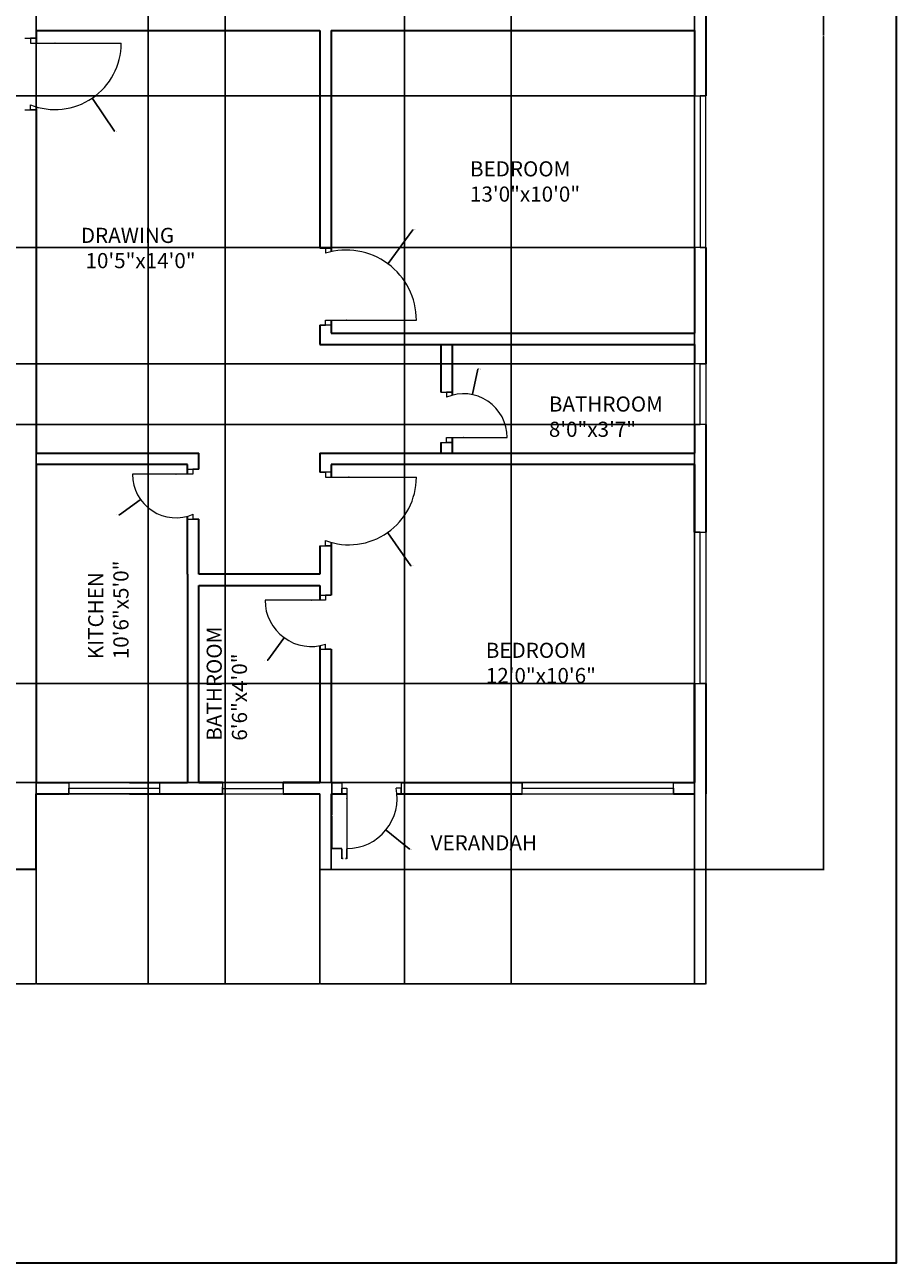
# Model space of a CAD drawing. Units: inches. Extents: x 1831 to 2867, y 1605 to 2524.
# Tile 6 of 7: x 2522 to 2867, y 1605 to 2096. Entities that reach past the tile are written whole.
import ezdxf

# ---------------------------------------------------------------- set-up
doc = ezdxf.new("R2010")
doc.units = ezdxf.units.IN
for name, color, linetype, lineweight in [('A-ANNO-DIMS', 2, 'Continuous', 18), ('A-ANNO-TTLB', 7, 'Continuous', 35), ('A-AREA-IDEN', 7, 'Continuous', 18), ('A-DOOR', 11, 'Continuous', 18), ('A-FLOR-BALC', 7, 'Continuous', 25), ('A-GLAZ', 121, 'Continuous', 18), ('A-WALL', 7, 'Continuous', 35)]:
    doc.layers.add(name, color=color, linetype=linetype, lineweight=lineweight)
doc.styles.get("Standard").update_dxf_attribs({"font": 'arial.ttf'})
doc.dimstyles.get("Standard").update_dxf_attribs({"dimtxt": 0.18, "dimasz": 0.18, "dimexe": 0.18, "dimexo": 0.0625, "dimgap": 0.09, "dimtad": 0, "dimtih": 1, "dimtoh": 1, "dimdec": 4, "dimzin": 0, "dimdsep": 46, "dimtxsty": 'Standard', "dimcen": 0.09, "dimadec": 0, "dimazin": 0, "dimtfac": 1, "dimtdec": 4, "dimtofl": 0, "dimtmove": 0, "dimatfit": 3, "dimfxl": 1, "dimtolj": 1, "dimtzin": 0, "dimarcsym": 0})

# ---------------------------------------------------------------- blocks, each defined once
blk = doc.blocks.new('WIN-60IN')
for p, q in [((4.5, 60), (0, 60)), ((0, 60), (2.25, 60)), ((0, 0), (0, 60)), ((2.25, 60), (2.25, 0)), ((4.5, 60), (4.5, 0)), ((4.5, 0), (0, 0)), ((2.25, 0), (4.5, 0))]:
    blk.add_line(p, q)
blk = doc.blocks.new('WIN-24IN')
for p, q in [((4.5, 24), (0, 24)), ((0, 24), (2.25, 24)), ((0, 0), (0, 24)), ((2.25, 24), (2.25, 0)), ((4.5, 0), (4.5, 24)), ((4.5, 0), (0, 0)), ((2.25, 0), (4.5, 0))]:
    blk.add_line(p, q)
blk = doc.blocks.new('WIN-60IN-ALT')
for p, q in [((0, 0), (0, 4.5)), ((0, 4.5), (0, 2.25)), ((60, 4.5), (0, 4.5)), ((0, 2.25), (60, 2.25)), ((0, 0), (60, 0)), ((60, 2.25), (60, 4.5)), ((60, 4.5), (60, 0))]:
    blk.add_line(p, q)
blk = doc.blocks.new('DOOR-LEAF-36IN')
for p, q in [((0, 2), (4.5, 2)), ((4.5, 2), (2.25, 2)), ((2.25, 2), (2.25, 0)), ((2.25, 0), (38.25, 0))]:
    blk.add_line(p, q)
blk = doc.blocks.new('DOOR-LEAF-36IN-ALT')
for p, q in [((36, 2), (0, 2)), ((33.75, 0), (38.25, 0)), ((36, 0), (36, 2)), ((38.25, 0), (36, 0))]:
    blk.add_line(p, q)
blk = doc.blocks.new('DOOR-LEAF-24IN')
for p, q in [((2.25, 0), (2.25, 2)), ((2.25, 2), (26.25, 2)), ((0, 0), (4.5, 0)), ((4.5, 0), (2.25, 0))]:
    blk.add_line(p, q)
blk = doc.blocks.new('DOOR-LEAF-24IN-ALT')
for p, q in [((24, 2), (0, 2)), ((21.75, 0), (26.25, 0)), ((24, 0), (24, 2)), ((26.25, 0), (24, 0))]:
    blk.add_line(p, q)
blk = doc.blocks.new('DOOR-STRIKE-JAMB')
for p, q in [((0, 0), (4.5, 0)), ((2.25, 0), (2.25, 2)), ((4.5, 0), (2.25, 0))]:
    blk.add_line(p, q)
blk = doc.blocks.new('*D14')
at = {"layer": 'A-ANNO-DIMS', "color": 0, "lineweight": -2, "transparency": 16777216}
for p, q in [((2647.23, 1795.67), (2643.17, 1795.67)), ((2643.35, 1795.49), (2643.35, 1782.73)), ((2643.35, 1769.6), (2643.35, 1782.37)), ((2647.23, 1769.42), (2643.17, 1769.42))]:
    blk.add_line(p, q, dxfattribs=at)
at = {"layer": 'A-ANNO-DIMS', "color": 0, "transparency": 16777216}
for points in [[(2643.32, 1795.49), (2643.38, 1795.49), (2643.35, 1795.67)], [(2643.32, 1769.6), (2643.38, 1769.6), (2643.35, 1769.42)]]:
    blk.add_solid(points, dxfattribs=at)
at = {"layer": 'Defpoints', "color": 0, "transparency": 16777216}
for p in [(2647.29, 1795.67), (2643.35, 1769.42), (2647.29, 1769.42)]:
    blk.add_point(p, dxfattribs=at)
at = {"layer": 'A-ANNO-DIMS', "color": 0, "transparency": 16777216, "insert": (2643.35, 1782.55), "char_height": 0.18, "attachment_point": 5}
blk.add_mtext('\\A1;DOOR LEAF 26 TYP.', dxfattribs=at)
blk = doc.blocks.new('*D15')
at = {"layer": 'A-ANNO-DIMS', "color": 0, "lineweight": -2, "transparency": 16777216}
for p, q in [((2647.29, 1769.36), (2647.29, 1765.31)), ((2649.29, 1769.36), (2649.29, 1765.31)), ((2647.47, 1765.49), (2647.83, 1765.49)), ((2649.11, 1765.49), (2648.75, 1765.49))]:
    blk.add_line(p, q, dxfattribs=at)
at = {"layer": 'A-ANNO-DIMS', "color": 0, "transparency": 16777216}
for points in [[(2647.47, 1765.52), (2647.47, 1765.46), (2647.29, 1765.49)], [(2649.11, 1765.52), (2649.11, 1765.46), (2649.29, 1765.49)]]:
    blk.add_solid(points, dxfattribs=at)
at = {"layer": 'Defpoints', "color": 0, "transparency": 16777216}
for p in [(2647.29, 1769.42), (2649.29, 1769.42), (2649.29, 1765.49)]:
    blk.add_point(p, dxfattribs=at)
at = {"layer": 'A-ANNO-DIMS', "color": 0, "transparency": 16777216, "insert": (2648.29, 1765.49), "char_height": 0.18, "attachment_point": 5}
blk.add_mtext('\\A1;2 TYP.', dxfattribs=at)
blk = doc.blocks.new('*D23')
at = {"layer": 'A-ANNO-DIMS', "color": 0, "lineweight": -2, "transparency": 16777216}
for p, q in [((2791.61, 2421.67), (2838.45, 2421.67)), ((2838.27, 2421.49), (2838.27, 2091.61)), ((2838.27, 1761.35), (2838.27, 2091.24)), ((2791.61, 1761.17), (2838.45, 1761.17))]:
    blk.add_line(p, q, dxfattribs=at)
at = {"layer": 'A-ANNO-DIMS', "color": 0, "transparency": 16777216}
for points in [[(2838.24, 2421.49), (2838.3, 2421.49), (2838.27, 2421.67)], [(2838.24, 1761.35), (2838.3, 1761.35), (2838.27, 1761.17)]]:
    blk.add_solid(points, dxfattribs=at)
at = {"layer": 'Defpoints', "color": 0, "transparency": 16777216}
for p in [(2791.55, 2421.67), (2838.27, 2421.67), (2791.55, 1761.17)]:
    blk.add_point(p, dxfattribs=at)
at = {"layer": 'A-ANNO-DIMS', "color": 0, "transparency": 16777216, "insert": (2838.27, 2091.42), "char_height": 0.18, "attachment_point": 5}
blk.add_mtext('\\A1;660.5', dxfattribs=at)
blk = doc.blocks.new('*D28')
at = {"layer": 'A-ANNO-DIMS', "color": 0, "lineweight": -2, "transparency": 16777216}
for p, q in [((2397.05, 1761.11), (2397.05, 1715.69)), ((2526.05, 1761.11), (2526.05, 1715.69)), ((2397.23, 1715.87), (2461.27, 1715.87)), ((2525.87, 1715.87), (2461.83, 1715.87))]:
    blk.add_line(p, q, dxfattribs=at)
at = {"layer": 'A-ANNO-DIMS', "color": 0, "transparency": 16777216}
for points in [[(2397.23, 1715.9), (2397.23, 1715.84), (2397.05, 1715.87)], [(2525.87, 1715.9), (2525.87, 1715.84), (2526.05, 1715.87)]]:
    blk.add_solid(points, dxfattribs=at)
at = {"layer": 'Defpoints', "color": 0, "transparency": 16777216}
for p in [(2397.05, 1761.17), (2526.05, 1761.17), (2526.05, 1715.87)]:
    blk.add_point(p, dxfattribs=at)
at = {"layer": 'A-ANNO-DIMS', "color": 0, "transparency": 16777216, "insert": (2461.55, 1715.87), "char_height": 0.18, "attachment_point": 5}
blk.add_mtext('\\A1;129', dxfattribs=at)
blk = doc.blocks.new('*D29')
at = {"layer": 'A-ANNO-DIMS', "color": 0, "lineweight": -2, "transparency": 16777216}
for p, q in [((2526.05, 1761.11), (2526.05, 1715.69)), ((2638.55, 1761.11), (2638.55, 1715.69)), ((2526.23, 1715.87), (2581.92, 1715.87)), ((2638.37, 1715.87), (2582.69, 1715.87))]:
    blk.add_line(p, q, dxfattribs=at)
at = {"layer": 'A-ANNO-DIMS', "color": 0, "transparency": 16777216}
for points in [[(2526.23, 1715.9), (2526.23, 1715.84), (2526.05, 1715.87)], [(2638.37, 1715.9), (2638.37, 1715.84), (2638.55, 1715.87)]]:
    blk.add_solid(points, dxfattribs=at)
at = {"layer": 'Defpoints', "color": 0, "transparency": 16777216}
for p in [(2526.05, 1761.17), (2638.55, 1761.17), (2638.55, 1715.87)]:
    blk.add_point(p, dxfattribs=at)
at = {"layer": 'A-ANNO-DIMS', "color": 0, "transparency": 16777216, "insert": (2582.3, 1715.87), "char_height": 0.18, "attachment_point": 5}
blk.add_mtext('\\A1;112.5', dxfattribs=at)
blk = doc.blocks.new('*D30')
at = {"layer": 'A-ANNO-DIMS', "color": 0, "lineweight": -2, "transparency": 16777216}
for p, q in [((2638.55, 1761.11), (2638.55, 1715.69)), ((2791.55, 1761.11), (2791.55, 1715.69)), ((2638.73, 1715.87), (2714.77, 1715.87)), ((2791.37, 1715.87), (2715.33, 1715.87))]:
    blk.add_line(p, q, dxfattribs=at)
at = {"layer": 'A-ANNO-DIMS', "color": 0, "transparency": 16777216}
for points in [[(2638.73, 1715.9), (2638.73, 1715.84), (2638.55, 1715.87)], [(2791.37, 1715.9), (2791.37, 1715.84), (2791.55, 1715.87)]]:
    blk.add_solid(points, dxfattribs=at)
at = {"layer": 'Defpoints', "color": 0, "transparency": 16777216}
for p in [(2638.55, 1761.17), (2791.55, 1761.17), (2791.55, 1715.87)]:
    blk.add_point(p, dxfattribs=at)
at = {"layer": 'A-ANNO-DIMS', "color": 0, "transparency": 16777216, "insert": (2715.05, 1715.87), "char_height": 0.18, "attachment_point": 5}
blk.add_mtext('\\A1;153', dxfattribs=at)
blk = doc.blocks.new('*D45')
at = {"layer": 'A-ANNO-DIMS', "color": 0, "lineweight": -2, "transparency": 16777216}
for p, q in [((2526.05, 2387.11), (2526.05, 1715.69)), ((2570.49, 2387.11), (2570.49, 1715.69)), ((2526.23, 1715.87), (2547.87, 1715.87)), ((2570.31, 1715.87), (2548.67, 1715.87))]:
    blk.add_line(p, q, dxfattribs=at)
at = {"layer": 'A-ANNO-DIMS', "color": 0, "transparency": 16777216}
for points in [[(2526.23, 1715.9), (2526.23, 1715.84), (2526.05, 1715.87)], [(2570.31, 1715.9), (2570.31, 1715.84), (2570.49, 1715.87)]]:
    blk.add_solid(points, dxfattribs=at)
at = {"layer": 'Defpoints', "color": 0, "transparency": 16777216}
for p in [(2526.05, 2387.17), (2570.49, 2387.17), (2570.49, 1715.87)]:
    blk.add_point(p, dxfattribs=at)
at = {"layer": 'A-ANNO-DIMS', "color": 0, "transparency": 16777216, "insert": (2548.27, 1715.87), "char_height": 0.18, "attachment_point": 5}
blk.add_mtext('\\A1;44.44', dxfattribs=at)
blk = doc.blocks.new('*D46')
at = {"layer": 'A-ANNO-DIMS', "color": 0, "lineweight": -2, "transparency": 16777216}
for p, q in [((2570.49, 2387.11), (2570.49, 1715.69)), ((2600.95, 2387.11), (2600.95, 1715.69)), ((2570.67, 1715.87), (2585.26, 1715.87)), ((2600.77, 1715.87), (2586.18, 1715.87))]:
    blk.add_line(p, q, dxfattribs=at)
at = {"layer": 'A-ANNO-DIMS', "color": 0, "transparency": 16777216}
for points in [[(2570.67, 1715.9), (2570.67, 1715.84), (2570.49, 1715.87)], [(2600.77, 1715.9), (2600.77, 1715.84), (2600.95, 1715.87)]]:
    blk.add_solid(points, dxfattribs=at)
at = {"layer": 'Defpoints', "color": 0, "transparency": 16777216}
for p in [(2570.49, 2387.17), (2600.95, 2387.17), (2600.95, 1715.87)]:
    blk.add_point(p, dxfattribs=at)
at = {"layer": 'A-ANNO-DIMS', "color": 0, "transparency": 16777216, "insert": (2585.72, 1715.87), "char_height": 0.18, "attachment_point": 5}
blk.add_mtext('\\A1;30.464', dxfattribs=at)
blk = doc.blocks.new('*D47')
at = {"layer": 'A-ANNO-DIMS', "color": 0, "lineweight": -2, "transparency": 16777216}
for p, q in [((2672.08, 2391.61), (2672.08, 1715.69)), ((2714.35, 2391.61), (2714.35, 1715.69)), ((2672.26, 1715.87), (2692.75, 1715.87)), ((2714.17, 1715.87), (2693.68, 1715.87))]:
    blk.add_line(p, q, dxfattribs=at)
at = {"layer": 'A-ANNO-DIMS', "color": 0, "transparency": 16777216}
for points in [[(2672.26, 1715.9), (2672.26, 1715.84), (2672.08, 1715.87)], [(2714.17, 1715.9), (2714.17, 1715.84), (2714.35, 1715.87)]]:
    blk.add_solid(points, dxfattribs=at)
at = {"layer": 'Defpoints', "color": 0, "transparency": 16777216}
for p in [(2672.08, 2391.67), (2714.35, 2391.67), (2714.35, 1715.87)]:
    blk.add_point(p, dxfattribs=at)
at = {"layer": 'A-ANNO-DIMS', "color": 0, "transparency": 16777216, "insert": (2693.22, 1715.87), "char_height": 0.18, "attachment_point": 5}
blk.add_mtext('\\A1;42.266', dxfattribs=at)
blk = doc.blocks.new('*D48')
at = {"layer": 'A-ANNO-DIMS', "color": 0, "lineweight": -2, "transparency": 16777216}
for p, q in [((2714.35, 2387.11), (2714.35, 1715.69)), ((2787.05, 2387.11), (2787.05, 1715.69)), ((2714.53, 1715.87), (2750.38, 1715.87)), ((2786.87, 1715.87), (2751.02, 1715.87))]:
    blk.add_line(p, q, dxfattribs=at)
at = {"layer": 'A-ANNO-DIMS', "color": 0, "transparency": 16777216}
for points in [[(2714.53, 1715.9), (2714.53, 1715.84), (2714.35, 1715.87)], [(2786.87, 1715.9), (2786.87, 1715.84), (2787.05, 1715.87)]]:
    blk.add_solid(points, dxfattribs=at)
at = {"layer": 'Defpoints', "color": 0, "transparency": 16777216}
for p in [(2714.35, 2387.17), (2787.05, 2387.17), (2787.05, 1715.87)]:
    blk.add_point(p, dxfattribs=at)
at = {"layer": 'A-ANNO-DIMS', "color": 0, "transparency": 16777216, "insert": (2750.7, 1715.87), "char_height": 0.18, "attachment_point": 5}
blk.add_mtext('\\A1;72.7', dxfattribs=at)
blk = doc.blocks.new('*D52')
at = {"layer": 'A-ANNO-DIMS', "color": 0, "lineweight": -2, "transparency": 16777216}
for p, q in [((2786.99, 2127.45), (1844.57, 2127.45)), ((1844.75, 2127.27), (1844.75, 2097.76)), ((1844.75, 2067.88), (1844.75, 2097.39)), ((2786.99, 2067.7), (1844.57, 2067.7))]:
    blk.add_line(p, q, dxfattribs=at)
at = {"layer": 'A-ANNO-DIMS', "color": 0, "transparency": 16777216}
for points in [[(1844.72, 2127.27), (1844.78, 2127.27), (1844.75, 2127.45)], [(1844.72, 2067.88), (1844.78, 2067.88), (1844.75, 2067.7)]]:
    blk.add_solid(points, dxfattribs=at)
at = {"layer": 'Defpoints', "color": 0, "transparency": 16777216}
for p in [(2787.05, 2127.45), (1844.75, 2067.7), (2787.05, 2067.7)]:
    blk.add_point(p, dxfattribs=at)
at = {"layer": 'A-ANNO-DIMS', "color": 0, "transparency": 16777216, "insert": (1844.75, 2097.57), "char_height": 0.18, "attachment_point": 5}
blk.add_mtext('\\A1;59.76', dxfattribs=at)
blk = doc.blocks.new('*D53')
at = {"layer": 'A-ANNO-DIMS', "color": 0, "lineweight": -2, "transparency": 16777216}
for p, q in [((2786.99, 2007.7), (1844.57, 2007.7)), ((1844.75, 2007.52), (1844.75, 1984.78)), ((1844.75, 1961.67), (1844.75, 1984.41)), ((2786.99, 1961.49), (1844.57, 1961.49))]:
    blk.add_line(p, q, dxfattribs=at)
at = {"layer": 'A-ANNO-DIMS', "color": 0, "transparency": 16777216}
for points in [[(1844.72, 2007.52), (1844.78, 2007.52), (1844.75, 2007.7)], [(1844.72, 1961.67), (1844.78, 1961.67), (1844.75, 1961.49)]]:
    blk.add_solid(points, dxfattribs=at)
at = {"layer": 'Defpoints', "color": 0, "transparency": 16777216}
for p in [(2787.05, 2007.7), (1844.75, 1961.49), (2787.05, 1961.49)]:
    blk.add_point(p, dxfattribs=at)
at = {"layer": 'A-ANNO-DIMS', "color": 0, "transparency": 16777216, "insert": (1844.75, 1984.59), "char_height": 0.18, "attachment_point": 5}
blk.add_mtext('\\A1;46.2', dxfattribs=at)
blk = doc.blocks.new('*D54')
at = {"layer": 'A-ANNO-DIMS', "color": 0, "lineweight": -2, "transparency": 16777216}
for p, q in [((2786.99, 1937.49), (1844.57, 1937.49)), ((1844.75, 1937.31), (1844.75, 1886.37)), ((1844.75, 1835.06), (1844.75, 1886)), ((2786.99, 1834.88), (1844.57, 1834.88))]:
    blk.add_line(p, q, dxfattribs=at)
at = {"layer": 'A-ANNO-DIMS', "color": 0, "transparency": 16777216}
for points in [[(1844.72, 1937.31), (1844.78, 1937.31), (1844.75, 1937.49)], [(1844.72, 1835.06), (1844.78, 1835.06), (1844.75, 1834.88)]]:
    blk.add_solid(points, dxfattribs=at)
at = {"layer": 'Defpoints', "color": 0, "transparency": 16777216}
for p in [(2787.05, 1937.49), (1844.75, 1834.88), (2787.05, 1834.88)]:
    blk.add_point(p, dxfattribs=at)
at = {"layer": 'A-ANNO-DIMS', "color": 0, "transparency": 16777216, "insert": (1844.75, 1886.19), "char_height": 0.18, "attachment_point": 5}
blk.add_mtext('\\A1;102.61', dxfattribs=at)
blk = doc.blocks.new('*D55')
at = {"layer": 'A-ANNO-DIMS', "color": 0, "lineweight": -2, "transparency": 16777216}
for p, q in [((2786.99, 1834.88), (1844.57, 1834.88)), ((1844.75, 1834.7), (1844.75, 1815.46)), ((1844.75, 1795.85), (1844.75, 1815.09)), ((2786.99, 1795.67), (1844.57, 1795.67))]:
    blk.add_line(p, q, dxfattribs=at)
at = {"layer": 'A-ANNO-DIMS', "color": 0, "transparency": 16777216}
for points in [[(1844.72, 1834.7), (1844.78, 1834.7), (1844.75, 1834.88)], [(1844.72, 1795.85), (1844.78, 1795.85), (1844.75, 1795.67)]]:
    blk.add_solid(points, dxfattribs=at)
at = {"layer": 'Defpoints', "color": 0, "transparency": 16777216}
for p in [(2787.05, 1834.88), (1844.75, 1795.67), (2787.05, 1795.67)]:
    blk.add_point(p, dxfattribs=at)
at = {"layer": 'A-ANNO-DIMS', "color": 0, "transparency": 16777216, "insert": (1844.75, 1815.28), "char_height": 0.18, "attachment_point": 5}
blk.add_mtext('\\A1;39.206', dxfattribs=at)
blk = doc.blocks.new('*D74')
at = {"layer": 'A-ANNO-DIMS', "color": 0, "lineweight": -2, "transparency": 16777216}
for p, q in [((2675.4, 2014.63), (2665.61, 2001.35)), ((2675.58, 2014.63), (2675.4, 2014.63)), ((2648.92, 1978.84), (2649.1, 1978.84)), ((2649.01, 1978.75), (2649.01, 1978.93))]:
    blk.add_line(p, q, dxfattribs=at)
at = {"layer": 'A-ANNO-DIMS', "color": 0, "transparency": 16777216}
blk.add_solid([(2665.59, 2001.37), (2665.64, 2001.34), (2665.51, 2001.21)], dxfattribs=at)
at = {"layer": 'Defpoints', "color": 0, "transparency": 16777216}
for p in [(2665.51, 2001.21), (2649.01, 1978.84)]:
    blk.add_point(p, dxfattribs=at)
at = {"layer": 'A-ANNO-DIMS', "color": 0, "transparency": 16777216, "insert": (2676.06, 2014.63), "char_height": 0.18, "attachment_point": 5}
blk.add_mtext('\\A1;R27.79', dxfattribs=at)
blk = doc.blocks.new('*D80')
at = {"layer": 'A-ANNO-DIMS', "color": 0, "lineweight": -2, "transparency": 16777216}
for p, q in [((2649.94, 1916.59), (2650.12, 1916.59)), ((2650.03, 1916.5), (2650.03, 1916.68)), ((2674.55, 1881.47), (2665.46, 1894.5)), ((2674.73, 1881.47), (2674.55, 1881.47))]:
    blk.add_line(p, q, dxfattribs=at)
at = {"layer": 'A-ANNO-DIMS', "color": 0, "transparency": 16777216}
blk.add_solid([(2665.48, 1894.51), (2665.43, 1894.48), (2665.35, 1894.64)], dxfattribs=at)
at = {"layer": 'Defpoints', "color": 0, "transparency": 16777216}
for p in [(2650.03, 1916.59), (2665.35, 1894.64)]:
    blk.add_point(p, dxfattribs=at)
at = {"layer": 'A-ANNO-DIMS', "color": 0, "transparency": 16777216, "insert": (2675.21, 1881.47), "char_height": 0.18, "attachment_point": 5}
blk.add_mtext('\\A1;R26.77', dxfattribs=at)
blk = doc.blocks.new('*D82')
at = {"layer": 'A-ANNO-DIMS', "color": 0, "lineweight": -2, "transparency": 16777216}
for p, q in [((2533.45, 2088.59), (2533.63, 2088.59)), ((2533.54, 2088.5), (2533.54, 2088.68)), ((2557.11, 2053.8), (2548.37, 2066.7)), ((2557.29, 2053.8), (2557.11, 2053.8))]:
    blk.add_line(p, q, dxfattribs=at)
at = {"layer": 'A-ANNO-DIMS', "color": 0, "transparency": 16777216}
blk.add_solid([(2548.39, 2066.72), (2548.35, 2066.68), (2548.27, 2066.85)], dxfattribs=at)
at = {"layer": 'Defpoints', "color": 0, "transparency": 16777216}
for p in [(2533.54, 2088.59), (2548.27, 2066.85)]:
    blk.add_point(p, dxfattribs=at)
at = {"layer": 'A-ANNO-DIMS', "color": 0, "transparency": 16777216, "insert": (2557.84, 2053.8), "char_height": 0.18, "attachment_point": 5}
blk.add_mtext('\\A1;R26.263', dxfattribs=at)
blk = doc.blocks.new('*D86')
at = {"layer": 'A-ANNO-DIMS', "color": 0, "lineweight": -2, "transparency": 16777216}
for p, q in [((2649.2, 1789.31), (2649.38, 1789.31)), ((2649.29, 1789.22), (2649.29, 1789.4)), ((2674.01, 1769.27), (2664.88, 1776.67)), ((2674.19, 1769.27), (2674.01, 1769.27))]:
    blk.add_line(p, q, dxfattribs=at)
at = {"layer": 'A-ANNO-DIMS', "color": 0, "transparency": 16777216}
blk.add_solid([(2664.9, 1776.7), (2664.86, 1776.65), (2664.74, 1776.79)], dxfattribs=at)
at = {"layer": 'Defpoints', "color": 0, "transparency": 16777216}
for p in [(2649.29, 1789.31), (2664.74, 1776.79)]:
    blk.add_point(p, dxfattribs=at)
at = {"layer": 'A-ANNO-DIMS', "color": 0, "transparency": 16777216, "insert": (2674.67, 1769.27), "char_height": 0.18, "attachment_point": 5}
blk.add_mtext('\\A1;R19.89', dxfattribs=at)
blk = doc.blocks.new('*D94')
at = {"layer": 'A-ANNO-DIMS', "color": 0, "lineweight": -2, "transparency": 16777216}
for p, q in [((2635.07, 1867.86), (2635.25, 1867.86)), ((2635.16, 1867.77), (2635.16, 1867.95)), ((2617.87, 1844.11), (2624.25, 1852.87)), ((2617.69, 1844.11), (2617.87, 1844.11))]:
    blk.add_line(p, q, dxfattribs=at)
at = {"layer": 'A-ANNO-DIMS', "color": 0, "transparency": 16777216}
blk.add_solid([(2624.23, 1852.89), (2624.27, 1852.85), (2624.36, 1853.01)], dxfattribs=at)
at = {"layer": 'Defpoints', "color": 0, "transparency": 16777216}
for p in [(2635.16, 1867.86), (2624.36, 1853.01)]:
    blk.add_point(p, dxfattribs=at)
at = {"layer": 'A-ANNO-DIMS', "color": 0, "transparency": 16777216, "insert": (2617.15, 1844.11), "char_height": 0.18, "attachment_point": 5}
blk.add_mtext('\\A1;R18.356', dxfattribs=at)
blk = doc.blocks.new('*D99')
at = {"layer": 'A-ANNO-DIMS', "color": 0, "lineweight": -2, "transparency": 16777216}
for p, q in [((2581.39, 1917.76), (2581.57, 1917.76)), ((2581.48, 1917.67), (2581.48, 1917.85)), ((2559.07, 1901.67), (2567.33, 1907.6)), ((2558.89, 1901.67), (2559.07, 1901.67))]:
    blk.add_line(p, q, dxfattribs=at)
at = {"layer": 'A-ANNO-DIMS', "color": 0, "transparency": 16777216}
blk.add_solid([(2567.31, 1907.63), (2567.35, 1907.58), (2567.48, 1907.71)], dxfattribs=at)
at = {"layer": 'Defpoints', "color": 0, "transparency": 16777216}
for p in [(2581.48, 1917.76), (2567.48, 1907.71)]:
    blk.add_point(p, dxfattribs=at)
at = {"layer": 'A-ANNO-DIMS', "color": 0, "transparency": 16777216, "insert": (2558.34, 1901.67), "char_height": 0.18, "attachment_point": 5}
blk.add_mtext('\\A1;R17.244', dxfattribs=at)
blk = doc.blocks.new('*D100')
at = {"layer": 'A-ANNO-DIMS', "color": 0, "lineweight": -2, "transparency": 16777216}
for p, q in [((2701.22, 1959.47), (2699.1, 1949.47)), ((2701.4, 1959.47), (2701.22, 1959.47)), ((2695.37, 1932.33), (2695.55, 1932.33)), ((2695.46, 1932.24), (2695.46, 1932.42))]:
    blk.add_line(p, q, dxfattribs=at)
at = {"layer": 'A-ANNO-DIMS', "color": 0, "transparency": 16777216}
blk.add_solid([(2699.07, 1949.48), (2699.13, 1949.46), (2699.06, 1949.29)], dxfattribs=at)
at = {"layer": 'Defpoints', "color": 0, "transparency": 16777216}
for p in [(2699.06, 1949.29), (2695.46, 1932.33)]:
    blk.add_point(p, dxfattribs=at)
at = {"layer": 'A-ANNO-DIMS', "color": 0, "transparency": 16777216, "insert": (2701.88, 1959.47), "char_height": 0.18, "attachment_point": 5}
blk.add_mtext('\\A1;R17.34', dxfattribs=at)

msp = doc.modelspace()

# ---------------------------------------------------------------- linework, layer by layer
at = {"layer": 'A-ANNO-TTLB'}
msp.add_lwpolyline([(1831.1248, 2523.9204), (2867.0416, 2523.9204), (2867.0416, 1605.0781), (1831.1248, 1605.0781)], close=True, dxfattribs=at)
at = {"layer": 'A-DOOR'}
for p, q in [((2526.051, 2062.2002), (2526.051, 2062.2002)), ((2586.051, 1919.763), (2589.2592, 1919.763)), ((2590.551, 1919.763), (2588.2405, 1919.763)), ((2588.2405, 1919.763), (2588.2405, 1917.763)), ((2589.2592, 1919.763), (2590.551, 1919.763)), ((2588.2405, 1917.763), (2564.2405, 1917.763))]:
    msp.add_line(p, q, dxfattribs=at)
for centre, radius, start, end in [((2533.5383, 2088.5911), 26.2627, 248.237268, 360), ((2649.0107, 1978.8425), 27.7903, 0, 107.182424), ((2695.4617, 1932.3313), 17.3393, 360, 112.590187), ((2581.4843, 1917.763), 17.2438, 180, 293.285515), ((2650.033, 1916.5931), 26.768, 249.825, 0), ((2635.1568, 1867.8551), 18.3558, 180, 287.907828), ((2649.2912, 1789.3129), 19.8892, 270, 11.928276)]:
    msp.add_arc(centre, radius, start, end, dxfattribs=at)
at = {"layer": 'A-FLOR-BALC'}
for p, q in [((2638.551, 1761.1738), (2638.551, 1791.1738)), ((2643.051, 1791.1738), (2643.051, 1761.1738)), ((2787.051, 1791.1738), (2787.051, 1773.1738)), ((2787.051, 1791.1738), (2787.051, 1761.1738)), ((2791.551, 1791.1738), (2791.551, 1773.1738)), ((2791.551, 1773.1738), (2791.551, 1761.1738)), ((2787.051, 1761.1738), (2638.551, 1761.1738)), ((2791.551, 1761.1738), (2787.051, 1761.1738))]:
    msp.add_line(p, q, dxfattribs=at)
at = {"layer": 'A-GLAZ'}
for p, q in [((2539.0573, 1795.6738), (2539.0573, 1791.1738)), ((2539.0573, 1795.6738), (2563.0573, 1795.6738)), ((2539.0573, 1791.1738), (2539.0573, 1793.4238)), ((2539.0573, 1793.4238), (2563.0573, 1793.4238)), ((2575.0573, 1795.6738), (2563.0573, 1795.6738)), ((2563.0573, 1793.4238), (2575.0573, 1793.4238)), ((2575.0573, 1791.1738), (2575.0573, 1795.6738)), ((2599.9742, 1795.6738), (2599.9742, 1792.0026)), ((2623.9742, 1795.6738), (2599.9742, 1795.6738)), ((2599.9742, 1791.1738), (2599.9742, 1793.8382)), ((2599.9742, 1793.8382), (2599.9742, 1793.2843)), ((2599.9742, 1793.2843), (2623.9742, 1793.2843)), ((2599.9742, 1792.0026), (2599.9742, 1791.1738)), ((2623.9742, 1793.2843), (2623.9742, 1795.6738)), ((2623.9742, 1795.6738), (2623.9742, 1791.1738)), ((2563.0573, 1791.1738), (2539.0573, 1791.1738)), ((2539.0573, 1791.1738), (2575.0573, 1791.1738)), ((2599.9742, 1791.1738), (2625.1892, 1791.1738))]:
    msp.add_line(p, q, dxfattribs=at)
at = {"layer": 'A-WALL'}
for p, q in [((2791.551, 2127.452), (2791.551, 2067.6955)), ((2526.051, 2093.6738), (2638.551, 2093.6738)), ((2526.051, 2093.6738), (2526.051, 2088.5911)), ((2638.551, 2093.6738), (2638.551, 2007.3925)), ((2643.051, 2093.6738), (2787.051, 2093.6738)), ((2643.051, 2093.6738), (2643.051, 2005.9862)), ((2787.051, 2093.6738), (2787.051, 2067.6955)), ((2526.051, 2063.4183), (2526.051, 1926.1738)), ((2787.051, 2007.6955), (2787.051, 1973.6738)), ((2791.551, 2007.6955), (2791.551, 1961.4909)), ((2643.051, 1978.8425), (2643.051, 1973.6738)), ((2638.551, 1976.8425), (2638.551, 1969.1738)), ((2643.051, 1973.6738), (2787.051, 1973.6738)), ((2638.551, 1969.1738), (2787.051, 1969.1738)), ((2686.551, 1969.1738), (2686.551, 1950.3402)), ((2691.051, 1969.1738), (2691.051, 1949.1002)), ((2787.051, 1969.1738), (2787.051, 1961.4909)), ((2787.051, 1937.4909), (2787.051, 1926.1738)), ((2791.551, 1937.4909), (2791.551, 1894.8797)), ((2686.551, 1930.3313), (2686.551, 1926.1738)), ((2691.051, 1932.3313), (2691.051, 1926.1738)), ((2526.051, 1926.1738), (2590.551, 1926.1738)), ((2590.551, 1919.763), (2590.551, 1926.1738)), ((2638.551, 1926.1738), (2787.051, 1926.1738)), ((2638.551, 1926.1738), (2638.551, 1918.5931)), ((2586.051, 1921.6738), (2526.051, 1921.6738)), ((2526.051, 1921.6738), (2526.051, 1795.6738)), ((2586.051, 1917.763), (2586.051, 1921.6738)), ((2787.051, 1921.6738), (2643.051, 1921.6738)), ((2643.051, 1921.6738), (2643.051, 1916.5931)), ((2787.051, 1921.6738), (2787.051, 1894.8797)), ((2787.051, 1894.8797), (2787.051, 1921.6738)), ((2586.051, 1878.1738), (2586.051, 1901.1349)), ((2590.551, 1878.1738), (2590.551, 1899.9238)), ((2643.051, 1890.7517), (2643.051, 1869.8551)), ((2638.551, 1889.4675), (2638.551, 1878.1738)), ((2586.051, 1878.1738), (2586.051, 1795.6738)), ((2638.551, 1878.1738), (2590.551, 1878.1738)), ((2590.551, 1795.6738), (2590.551, 1873.6738)), ((2590.551, 1873.6738), (2638.551, 1873.6738)), ((2638.551, 1873.6738), (2638.551, 1867.8551)), ((2638.551, 1849.8158), (2638.551, 1795.6738)), ((2643.051, 1848.3886), (2643.051, 1795.6738)), ((2787.051, 1795.6738), (2787.051, 1834.8797)), ((2787.051, 1834.8797), (2787.051, 1795.6738)), ((2791.551, 1834.8797), (2791.551, 1791.1738)), ((2526.051, 1795.6738), (2539.0573, 1795.6738)), ((2563.0573, 1795.6738), (2586.051, 1795.6738)), ((2590.551, 1795.6738), (2599.9742, 1795.6738)), ((2599.9742, 1795.6738), (2590.551, 1795.6738)), ((2638.551, 1795.6738), (2623.9742, 1795.6738)), ((2623.9742, 1795.6738), (2638.551, 1795.6738)), ((2643.051, 1795.6738), (2647.2912, 1795.6738)), ((2670.7509, 1795.6738), (2718.7347, 1795.6738)), ((2778.7347, 1795.6738), (2787.051, 1795.6738)), ((2526.051, 1761.1738), (2526.051, 1791.1738)), ((2526.051, 1791.1738), (2539.0573, 1791.1738)), ((2563.0573, 1791.1738), (2599.9742, 1791.1738)), ((2623.9742, 1791.1738), (2638.551, 1791.1738)), ((2643.051, 1791.1738), (2649.2912, 1791.1738)), ((2669.0932, 1791.1738), (2718.7347, 1791.1738)), ((2778.7347, 1791.1738), (2787.051, 1791.1738)), ((2526.051, 1761.1738), (2481.4899, 1761.1738))]:
    msp.add_line(p, q, dxfattribs=at)

# ---------------------------------------------------------------- block references
at = {"layer": 'A-DOOR'}
for name, p in [('DOOR-LEAF-36IN', (2521.551, 2088.5911)), ('DOOR-STRIKE-JAMB', (2521.551, 2062.2002)), ('DOOR-LEAF-24IN', (2686.551, 1930.3313)), ('DOOR-STRIKE-JAMB', (2586.051, 1899.9238)), ('DOOR-STRIKE-JAMB', (2638.551, 1889.4675)), ('DOOR-STRIKE-JAMB', (2638.551, 1848.3886))]:
    msp.add_blockref(name, p, dxfattribs=at)
at = {"layer": 'A-DOOR', "extrusion": (0, 0, -1), "zscale": -1}
for name, p, rotation in [('DOOR-STRIKE-JAMB', (-2638.551, 2007.3925), 180), ('DOOR-STRIKE-JAMB', (-2686.551, 1950.3402), 180), ('DOOR-LEAF-24IN-ALT', (-2616.801, 1869.8551), 180), ('DOOR-STRIKE-JAMB', (-2670.7509, 1795.6738), 270.0000000000085)]:
    msp.add_blockref(name, p, dxfattribs=dict(at, rotation=rotation))
msp.add_blockref('DOOR-LEAF-36IN-ALT', (-2676.801, 1976.8425), dxfattribs=at)
at = {"layer": 'A-DOOR'}
for name, p, rotation in [('DOOR-LEAF-36IN-ALT', (2676.801, 1918.5931), 180), ('DOOR-LEAF-24IN', (2647.2912, 1795.6738), 269.9999999999985)]:
    msp.add_blockref(name, p, dxfattribs=dict(at, rotation=rotation))
at = {"layer": 'A-GLAZ'}
for name, p, rotation in [('WIN-60IN-ALT', (2787.051, 2067.6955), 269.9999999999998), ('WIN-60IN', (2791.551, 1894.8797), 180)]:
    msp.add_blockref(name, p, dxfattribs=dict(at, rotation=rotation))
at = {"layer": 'A-GLAZ', "extrusion": (0, 0, -1), "zscale": -1}
for name, p, rotation in [('WIN-24IN', (-2787.051, 1961.4909), 180), ('WIN-60IN', (-2778.7347, 1795.6738), 269.9999999999988)]:
    msp.add_blockref(name, p, dxfattribs=dict(at, rotation=rotation))

# ---------------------------------------------------------------- texts
at = {"layer": 'A-AREA-IDEN', "char_height": 6, "attachment_point": 1}
for s, width, insert in [('BEDROOM\\P13\'0"x10\'0"', 118.828647, (2698.0607, 2041.8198)), ('DRAWING\\P 10\'5"x14\'0"', 177.829253, (2543.7965, 2015.4476)), ('BATHROOM\\P8\'0"x3\'7"', 95.886328, (2729.3299, 1948.6088)), ('BEDROOM\\P12\'0"x10\'6"', 133.649326, (2704.3275, 1851.0015)), ('VERANDAH', 121.894867, (2682.4529, 1774.6941))]:
    msp.add_mtext_dynamic_manual_height_columns(s, width=width, gutter_width=12.5, heights=[0], dxfattribs=dict(at, insert=insert))
at = {"layer": 'A-AREA-IDEN', "char_height": 6, "attachment_point": 1, "rotation": 90}
for s, width, insert in [('KITCHEN\\P10\'6"x5\'0"', 151.051789, (2546.6758, 1844.4666)), ('BATHROOM\\P6\'6"x4\'0"', 93.191719, (2593.6614, 1812.1792))]:
    msp.add_mtext_dynamic_manual_height_columns(s, width=width, gutter_width=12.5, heights=[0], dxfattribs=dict(at, insert=insert))

# ---------------------------------------------------------------- dimensions: what is measured, and where the dimension line sits
at = {"layer": 'A-ANNO-DIMS'}
for base, p1, p2, override, picture, middle in [((2838.2663, 2421.6738), (2791.551, 1761.1738), (2791.551, 2421.6738), {"dimdec": 1, "dimlfac": 1, "dimrnd": 0, "dimzin": 0, "dimdsep": 46, "dimlunit": 2}, '*D23', (2838.2663, 2091.4238)), ((1844.751, 2067.6955), (2787.051, 2127.452), (2787.051, 2067.6955), {"dimdec": 2, "dimlfac": 1, "dimrnd": 0, "dimzin": 0, "dimdsep": 46, "dimlunit": 2}, '*D52', (1844.751, 2097.5738)), ((1844.751, 1961.4909), (2787.051, 2007.6955), (2787.051, 1961.4909), {"dimdec": 1, "dimlfac": 1, "dimrnd": 0, "dimzin": 0, "dimdsep": 46, "dimlunit": 2}, '*D53', (1844.751, 1984.5932)), ((1844.751, 1834.8797), (2787.051, 1937.4909), (2787.051, 1834.8797), {"dimdec": 2, "dimlfac": 1, "dimrnd": 0, "dimzin": 0, "dimdsep": 46, "dimlunit": 2}, '*D54', (1844.751, 1886.1853)), ((1844.751, 1795.6738), (2787.051, 1834.8797), (2787.051, 1795.6738), {"dimdec": 3, "dimlfac": 1, "dimrnd": 0, "dimzin": 0, "dimdsep": 46, "dimlunit": 2}, '*D55', (1844.751, 1815.2767))]:
    dim = msp.add_linear_dim(base=base, p1=p1, p2=p2, angle=90, dimstyle='Standard', override=override, dxfattribs=at)
    dim.commit()
    dim.dimension.update_dxf_attribs({"geometry": picture, "text_midpoint": middle})
for base, p1, p2, override, picture, middle in [((2714.3491, 1715.8738), (2672.0835, 2391.6738), (2714.3491, 2391.6738), {"dimdec": 3, "dimlfac": 1, "dimrnd": 0, "dimzin": 0, "dimdsep": 46, "dimlunit": 2}, '*D47', (2693.2163, 1715.8738)), ((2570.4894, 1715.8738), (2526.051, 2387.1738), (2570.4894, 2387.1738), {"dimdec": 2, "dimlfac": 1, "dimrnd": 0, "dimzin": 0, "dimdsep": 46, "dimlunit": 2}, '*D45', (2548.2702, 1715.8738)), ((2600.9537, 1715.8738), (2570.4894, 2387.1738), (2600.9537, 2387.1738), {"dimdec": 3, "dimlfac": 1, "dimrnd": 0, "dimzin": 0, "dimdsep": 46, "dimlunit": 2}, '*D46', (2585.7216, 1715.8738)), ((2787.051, 1715.8738), (2714.3491, 2387.1738), (2787.051, 2387.1738), {"dimdec": 1, "dimlfac": 1, "dimrnd": 0, "dimzin": 0, "dimdsep": 46, "dimlunit": 2}, '*D48', (2750.7001, 1715.8738)), ((2526.051, 1715.8738), (2397.051, 1761.1738), (2526.051, 1761.1738), {"dimdec": 0, "dimlfac": 1, "dimrnd": 0, "dimzin": 0, "dimdsep": 46, "dimlunit": 2}, '*D28', (2461.551, 1715.8738)), ((2638.551, 1715.8738), (2526.051, 1761.1738), (2638.551, 1761.1738), {"dimdec": 1, "dimlfac": 1, "dimrnd": 0, "dimzin": 0, "dimdsep": 46, "dimlunit": 2}, '*D29', (2582.301, 1715.8738)), ((2791.551, 1715.8738), (2638.551, 1761.1738), (2791.551, 1761.1738), {"dimdec": 0, "dimlfac": 1, "dimrnd": 0, "dimzin": 0, "dimdsep": 46, "dimlunit": 2}, '*D30', (2715.051, 1715.8738))]:
    dim = msp.add_linear_dim(base=base, p1=p1, p2=p2, dimstyle='Standard', override=override, dxfattribs=at)
    dim.commit()
    dim.dimension.update_dxf_attribs({"geometry": picture, "text_midpoint": middle})
for center, mpoint, override, picture, middle in [((2533.5383, 2088.5911), (2548.2692, 2066.8487), {"dimdec": 3, "dimlfac": 1, "dimrnd": 0, "dimzin": 0, "dimdsep": 46, "dimlunit": 2}, '*D82', (2557.8375, 2053.8033)), ((2649.0107, 1978.8425), (2665.5052, 2001.2083), {"dimdec": 2, "dimlfac": 1, "dimrnd": 0, "dimzin": 0, "dimdsep": 46, "dimlunit": 2}, '*D74', (2676.062, 2014.6278)), ((2695.4617, 1932.3313), (2699.059, 1949.2933), {"dimdec": 2, "dimlfac": 1, "dimrnd": 0, "dimzin": 0, "dimdsep": 46, "dimlunit": 2}, '*D100', (2701.8768, 1959.4706)), ((2581.4843, 1917.763), (2567.4767, 1907.7063), {"dimdec": 3, "dimlfac": 1, "dimrnd": 0, "dimzin": 0, "dimdsep": 46, "dimlunit": 2}, '*D99', (2558.3427, 1901.6723)), ((2650.033, 1916.5931), (2665.3532, 1894.6428), {"dimdec": 2, "dimlfac": 1, "dimrnd": 0, "dimzin": 0, "dimdsep": 46, "dimlunit": 2}, '*D80', (2675.2051, 1881.4725)), ((2635.1568, 1867.8551), (2624.3557, 1853.0136), {"dimdec": 3, "dimlfac": 1, "dimrnd": 0, "dimzin": 0, "dimdsep": 46, "dimlunit": 2}, '*D94', (2617.1453, 1844.1086)), ((2649.2912, 1789.3129), (2664.7403, 1776.7868), {"dimdec": 2, "dimlfac": 1, "dimrnd": 0, "dimzin": 0, "dimdsep": 46, "dimlunit": 2}, '*D86', (2674.6698, 1769.271))]:
    dim = msp.add_radius_dim(center=center, mpoint=mpoint, dimstyle='Standard', override=override, dxfattribs=at)
    dim.commit()
    dim.dimension.update_dxf_attribs({"geometry": picture, "text_midpoint": middle, "dimtype": 164})
dim = msp.add_linear_dim(base=(2643.3537, 1769.4238), p1=(2647.2912, 1795.6738), p2=(2647.2912, 1769.4238), angle=270, text='DOOR LEAF <> TYP.', dimstyle='Standard', override={"dimdec": 0, "dimlfac": 1, "dimrnd": 0, "dimzin": 0, "dimdsep": 46, "dimlunit": 2}, dxfattribs=at)
dim.commit()
dim.dimension.update_dxf_attribs({"geometry": '*D14', "text_midpoint": (2643.3537, 1782.5488)})
dim = msp.add_linear_dim(base=(2649.2912, 1765.4863), p1=(2647.2912, 1769.4238), p2=(2649.2912, 1769.4238), text='<> TYP.', dimstyle='Standard', override={"dimdec": 0, "dimlfac": 1, "dimrnd": 0, "dimzin": 0, "dimdsep": 46, "dimlunit": 2}, dxfattribs=at)
dim.commit()
dim.dimension.update_dxf_attribs({"geometry": '*D15', "text_midpoint": (2648.2912, 1765.4863)})

doc.saveas('drawing.dxf')
